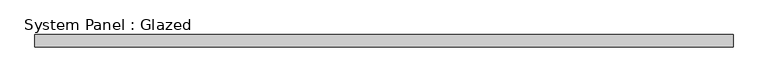
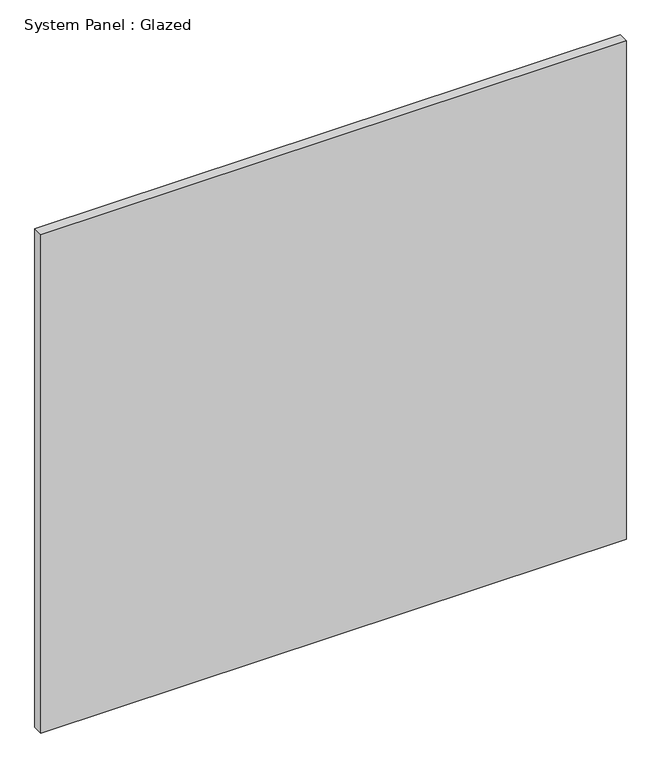
"""IFC4 building model written with IfcOpenShell, lengths in millimetres: plate geometry, System Panel : Glazed."""

from ifc_helpers import new_model, si_unit, origin, origin_with_axes, place, context, project, spatial, polyline, outline, extrude, source, transform, mapped, element, save


def system_panel_glazed_ae745dbd(model_context):
    return source(origin(), model_context, "Body", "SweptSolid", [
        extrude(outline(polyline([(711.2, 19.05), (-711.2, 19.05), (-711.2, 44.45), (711.2, 44.45), (711.2, 19.05)])), origin_with_axes(), (0.0, 0.0, 1.0), 1279.4174829),
    ])


if __name__ == "__main__":
    model = new_model("IFC4")
    model_context = context("Model", 3, world=origin())
    ifc_project = project(units=[si_unit("LENGTHUNIT", "METRE", prefix="MILLI")], contexts=[model_context])
    site = spatial("IfcSite", under=ifc_project)
    building = spatial("IfcBuilding", under=site)
    placement = place(None, origin())
    system_panel_glazed_shape = system_panel_glazed_ae745dbd(model_context)
    element("IfcPlate", 1, ObjectType="System Panel : Glazed", at=placement, inside=building, context=model_context, shape_type="MappedRepresentation", body=[
        mapped(system_panel_glazed_shape, transform((0.0, 0.0, 0.0), x_axis=(1.0, 0.0, 0.0), y_axis=(0.0, 1.0, 0.0), z_axis=(0.0, 0.0, 1.0))),
    ])
    save(model, "model.ifc")

# Revit data of these elements
# Type "System Panel : Glazed"
#   Construction Type Id = "GSP4R"
#   Analytic Construction = "1/8 in Pilkington single glazing"
#   Visual Light Transmittance = 0.9
#   Solar Heat Gain Coefficient = 0.86
#   Heat Transfer Coefficient (U) = 1.18115 BTU/(h·ft²·°F)
#   Define Thermal Properties by = 1
# Element 1 (IfcPlate, "System Panel : Glazed")
#   Materials on its faces: "Glass"
# Materials
#   "Glass": class "Glass", colour RGB 0 128 192, transparency 0.75, Description = "Soda Lime Glass", Cost = 0
